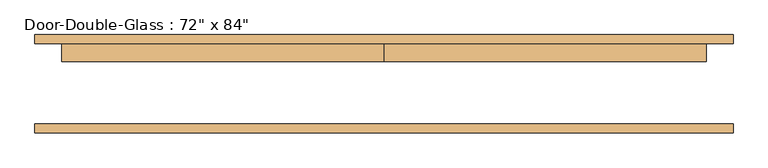
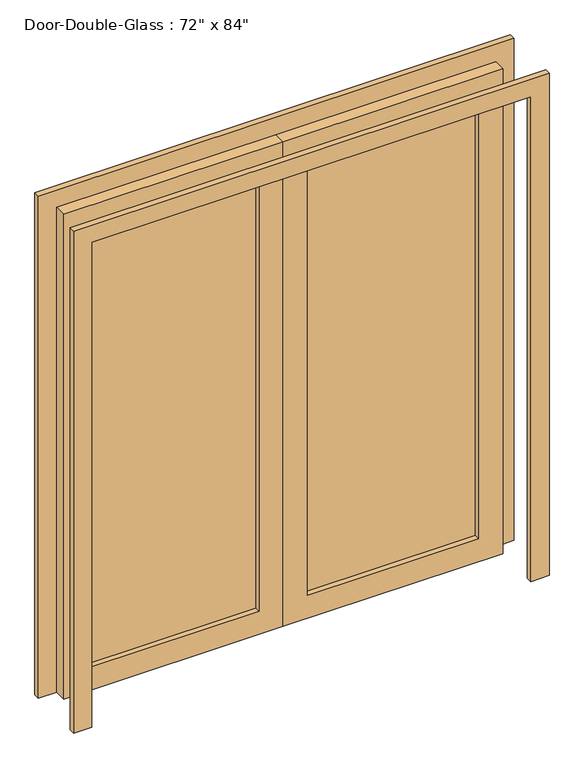
"""IFC4 building model written with IfcOpenShell, lengths in millimetres: door geometry."""

from ifc_helpers import new_model, si_unit, frame, origin, place, context, project, spatial, polyline, outline, extrude, source, transform, mapped, element, save


def door_5cbd26dd(model_context):
    return source(origin(), model_context, "Body", "SweptSolid", [
        extrude(outline(polyline([(2133.6, 914.4), (2133.6, 0.0), (0.0, 0.0), (0.0, 914.4), (2133.6, 914.4)]), holes=[polyline([(2032.0, 812.8), (101.6, 812.8), (101.6, 101.6), (2032.0, 101.6), (2032.0, 812.8)])]), frame((0.0, 65.88125, 0.0), z_axis=(0.0, 1.0, 0.0), x_axis=(0.0, 0.0, 1.0)), (0.0, 0.0, 1.0), 50.8),
        extrude(outline(polyline([(2133.6, -914.4), (0.0, -914.4), (0.0, 0.0), (2133.6, 0.0), (2133.6, -914.4)]), holes=[polyline([(2032.0, -812.8), (2032.0, -101.6), (101.6, -101.6), (101.6, -812.8), (2032.0, -812.8)])]), frame((0.0, 65.88125, 0.0), z_axis=(0.0, 1.0, 0.0), x_axis=(0.0, 0.0, 1.0)), (0.0, 0.0, 1.0), 50.8),
        extrude(outline(polyline([(-812.8, 94.45625), (-101.6, 94.45625), (-101.6, 88.10625), (-812.8, 88.10625), (-812.8, 94.45625)])), frame((0.0, 0.0, 101.6), z_axis=(0.0, 0.0, 1.0), x_axis=(1.0, 0.0, 0.0)), (0.0, 0.0, 1.0), 1930.4),
        extrude(outline(polyline([(101.6, 94.45625), (812.8, 94.45625), (812.8, 88.10625), (101.6, 88.10625), (101.6, 94.45625)])), frame((0.0, 0.0, 101.6), z_axis=(0.0, 0.0, 1.0), x_axis=(1.0, 0.0, 0.0)), (0.0, 0.0, 1.0), 1930.4),
        extrude(outline(polyline([(0.0, 990.6), (2209.8, 990.6), (2209.8, -990.6), (0.0, -990.6), (0.0, -914.4), (2133.6, -914.4), (2133.6, 914.4), (0.0, 914.4), (0.0, 990.6)])), frame((0.0, -137.31875, 0.0), z_axis=(0.0, 1.0, 0.0), x_axis=(0.0, 0.0, 1.0)), (0.0, 0.0, 1.0), 25.4),
        extrude(outline(polyline([(0.0, 990.6), (2209.8, 990.6), (2209.8, -990.6), (0.0, -990.6), (0.0, -914.4), (2133.6, -914.4), (2133.6, 914.4), (0.0, 914.4), (0.0, 990.6)])), frame((0.0, 116.68125, 0.0), z_axis=(0.0, 1.0, 0.0), x_axis=(0.0, 0.0, 1.0)), (0.0, 0.0, 1.0), 25.4),
    ])


if __name__ == "__main__":
    model = new_model("IFC4")
    model_context = context("Model", 3, world=origin())
    ifc_project = project(units=[si_unit("LENGTHUNIT", "METRE", prefix="MILLI")], contexts=[model_context])
    site = spatial("IfcSite", under=ifc_project)
    building = spatial("IfcBuilding", under=site)
    placement = place(None, origin())
    door_shape = door_5cbd26dd(model_context)
    element("IfcDoor", 1, ObjectType="Door-Double-Glass : 72\" x 84\"", at=placement, inside=building, context=model_context, shape_type="MappedRepresentation", body=[
        mapped(door_shape, transform((0.0, 0.0, 0.0), x_axis=(1.0, 0.0, 0.0), y_axis=(0.0, 1.0, 0.0), z_axis=(0.0, 0.0, 1.0))),
    ])
    save(model, "model.ifc")

# Revit data of these elements
# Type "Door-Double-Glass : 72\" x 84\""
#   Type Mark = "13"
#   Construction Type Id = "opn-d45"
#   Assembly Code = "C1020"
#   Analytic Construction = "Wood frame, double glass door "
#   W = 3' - 0"
#   Thickness = 0' - 2"
#   Thermal Resistance (R) = 1.8150 (h·ft²·°F)/BTU
#   Swing Angle [instance default] = 90.00°
#   Heat Transfer Coefficient (U) = 0.5510 BTU/(h·ft²·°F)
#   Height = 7' - 0"
#   Bottom Rail = 0' - 4"
#   Top Rail = 0' - 4"
#   Stiles = 0' - 4"
#   Trim Projection = 0' - 1"
#   Trim Width = 0' - 3"
#   Width = 6' - 0"
#   Define Thermal Properties by = 1
#   Glazing = Glass
#   Panel Material = Wood - Birch - Solid Stained Light Low Gloss
#   Trim Material = Paint - Sienna
#   Visual Light Transmittance = 0
#   Solar Heat Gain Coefficient = 0
#   Function = (empty or 0)
#   Wall Closure = (empty or 0)
# Element 1 (IfcDoor, "Door-Double-Glass : 72\" x 84\"")
#   Materials on its faces: "Wood - Birch - Solid Stained Light Low Gloss", "Paint - Sienna", "Glass"
# Materials
#   "Glass": class "Glass", colour RGB 0 128 192, transparency 0.75, Description = "Soda Lime Glass", Cost = 0
#   "Wood - Birch - Solid Stained Light Low Gloss": class "Wood", colour RGB 210 159 95, transparency 0, Cost = 0
#   "Paint - Sienna": colour RGB 118 70 51, transparency 0, Cost = 0
